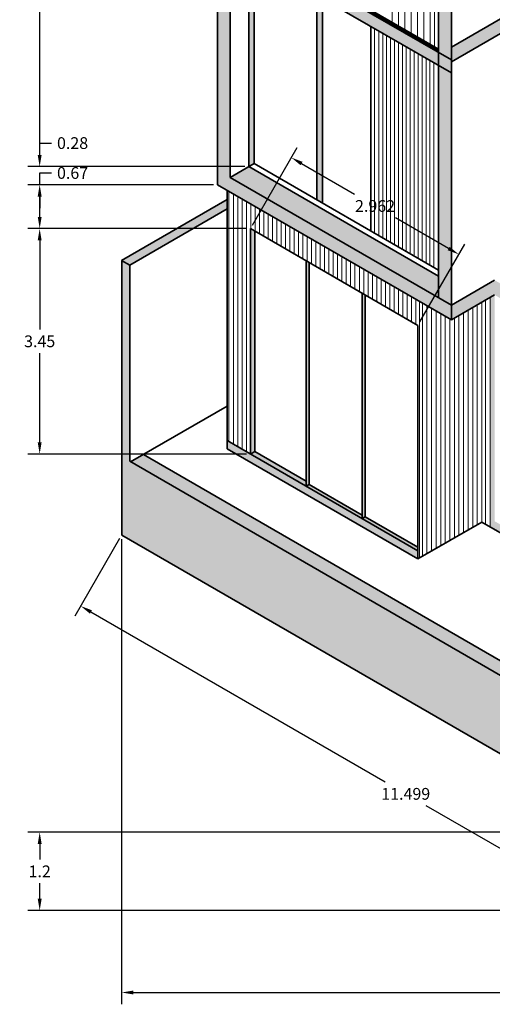
# Model space of a CAD drawing. Units: metres. Extents: x 26125 to 52281, y 14233 to 28508.
# Tile 1 of 4: x 26125.05 to 26132.29, y 14233.46 to 14248.53. Entities that reach past the tile are written whole.
import ezdxf

# ---------------------------------------------------------------- set-up
doc = ezdxf.new("R2010")
doc.units = ezdxf.units.M
for name, color, linetype, lineweight in [('A-ANNO-DIMS', 2, 'Continuous', 18), ('A-ELEV', 7, 'Continuous', 18), ('A-ELEV-CLAD', 30, 'Continuous', 13), ('A-ELEV-PATT', 32, 'Continuous', 13), ('A-WALL', 7, 'Continuous', 35), ('A-WALL-PATT', 9, 'Continuous', 13)]:
    doc.layers.add(name, color=color, linetype=linetype, lineweight=lineweight)
doc.styles.get("Standard").update_dxf_attribs({"font": 'arial.ttf'})
doc.dimstyles.get("Standard").update_dxf_attribs({"dimtxt": 0.18, "dimasz": 0.18, "dimexe": 0.18, "dimexo": 0.0625, "dimgap": 0.09, "dimtad": 0, "dimtih": 1, "dimtoh": 1, "dimdec": 4, "dimzin": 0, "dimdsep": 46, "dimtxsty": 'Standard', "dimcen": 0.09, "dimadec": 0, "dimazin": 0, "dimtfac": 1, "dimtdec": 4, "dimtofl": 0, "dimtmove": 0, "dimatfit": 3, "dimfxl": 1, "dimtolj": 1, "dimtzin": 0, "dimarcsym": 0})

# ---------------------------------------------------------------- blocks, each defined once
blk = doc.blocks.new('*D10')
at = {"layer": 'A-ANNO-DIMS', "color": 0, "lineweight": -2, "transparency": 16777216}
for p, q in [((26148.791, 14241.887), (26148.791, 14233.458)), ((26126.609, 14240.579), (26126.609, 14233.458)), ((26126.789, 14233.638), (26137.305, 14233.638)), ((26148.611, 14233.638), (26138.096, 14233.638))]:
    blk.add_line(p, q, dxfattribs=at)
at = {"layer": 'A-ANNO-DIMS', "color": 0, "transparency": 16777216}
for points in [[(26126.789, 14233.668), (26126.789, 14233.608), (26126.609, 14233.638)], [(26148.611, 14233.668), (26148.611, 14233.608), (26148.791, 14233.638)]]:
    blk.add_solid(points, dxfattribs=at)
at = {"layer": 'Defpoints', "color": 0, "transparency": 16777216}
for p in [(26148.791, 14241.95), (26126.609, 14240.642), (26148.791, 14233.638)]:
    blk.add_point(p, dxfattribs=at)
at = {"layer": 'A-ANNO-DIMS', "color": 0, "transparency": 16777216, "insert": (26137.7, 14233.638), "char_height": 0.18, "attachment_point": 5}
blk.add_mtext('\\A1;22.18', dxfattribs=at)
blk = doc.blocks.new('*D12')
at = {"layer": 'A-ANNO-DIMS', "color": 0, "lineweight": -2, "transparency": 16777216}
for p, q in [((26126.578, 14240.588), (26125.892, 14239.399)), ((26126.138, 14239.465), (26130.646, 14236.862)), ((26135.784, 14233.896), (26131.276, 14236.498)), ((26136.536, 14234.838), (26135.85, 14233.65))]:
    blk.add_line(p, q, dxfattribs=at)
at = {"layer": 'A-ANNO-DIMS', "color": 0, "transparency": 16777216}
for points in [[(26126.153, 14239.491), (26126.123, 14239.439), (26125.982, 14239.555)], [(26135.799, 14233.922), (26135.769, 14233.87), (26135.94, 14233.806)]]:
    blk.add_solid(points, dxfattribs=at)
at = {"layer": 'Defpoints', "color": 0, "transparency": 16777216}
for p in [(26126.609, 14240.642), (26125.982, 14239.555), (26136.568, 14234.893)]:
    blk.add_point(p, dxfattribs=at)
at = {"layer": 'A-ANNO-DIMS', "color": 0, "transparency": 16777216, "insert": (26130.961, 14236.68), "char_height": 0.18, "attachment_point": 5}
blk.add_mtext('\\A1;11.499', dxfattribs=at)
blk = doc.blocks.new('*D14')
at = {"layer": 'A-ANNO-DIMS', "color": 0, "lineweight": -2, "transparency": 16777216}
for p, q in [((26136.505, 14236.093), (26125.173, 14236.093)), ((26125.353, 14235.913), (26125.353, 14235.673)), ((26125.353, 14235.073), (26125.353, 14235.312)), ((26136.505, 14234.893), (26125.173, 14234.893))]:
    blk.add_line(p, q, dxfattribs=at)
at = {"layer": 'A-ANNO-DIMS', "color": 0, "transparency": 16777216}
for points in [[(26125.323, 14235.913), (26125.383, 14235.913), (26125.353, 14236.093)], [(26125.323, 14235.073), (26125.383, 14235.073), (26125.353, 14234.893)]]:
    blk.add_solid(points, dxfattribs=at)
at = {"layer": 'Defpoints', "color": 0, "transparency": 16777216}
for p in [(26125.353, 14236.093), (26136.568, 14236.093), (26136.568, 14234.893)]:
    blk.add_point(p, dxfattribs=at)
at = {"layer": 'A-ANNO-DIMS', "color": 0, "transparency": 16777216, "insert": (26125.353, 14235.493), "char_height": 0.18, "attachment_point": 5}
blk.add_mtext('\\A1;1.2', dxfattribs=at)
blk = doc.blocks.new('*D23')
at = {"layer": 'A-ANNO-DIMS', "color": 0, "lineweight": -2, "transparency": 16777216}
for p, q in [((26128.519, 14245.334), (26125.173, 14245.334)), ((26125.353, 14245.154), (26125.353, 14243.791)), ((26125.353, 14242.063), (26125.353, 14243.427)), ((26128.519, 14241.883), (26125.173, 14241.883))]:
    blk.add_line(p, q, dxfattribs=at)
at = {"layer": 'A-ANNO-DIMS', "color": 0, "transparency": 16777216}
for points in [[(26125.323, 14245.154), (26125.383, 14245.154), (26125.353, 14245.334)], [(26125.323, 14242.063), (26125.383, 14242.063), (26125.353, 14241.883)]]:
    blk.add_solid(points, dxfattribs=at)
at = {"layer": 'Defpoints', "color": 0, "transparency": 16777216}
for p in [(26125.353, 14245.334), (26128.581, 14245.334), (26128.581, 14241.883)]:
    blk.add_point(p, dxfattribs=at)
at = {"layer": 'A-ANNO-DIMS', "color": 0, "transparency": 16777216, "insert": (26125.353, 14243.609), "char_height": 0.18, "attachment_point": 5}
blk.add_mtext('\\A1;3.45', dxfattribs=at)
blk = doc.blocks.new('*D24')
at = {"layer": 'A-ANNO-DIMS', "color": 0, "lineweight": -2, "transparency": 16777216}
for p, q in [((26125.35337, 14246.006223), (26125.35337, 14246.186223)), ((26125.35337, 14246.186223), (26125.53337, 14246.186223)), ((26128.013551, 14246.006223), (26125.17337, 14246.006223)), ((26125.35337, 14245.514375), (26125.35337, 14245.826223)), ((26128.518849, 14245.334375), (26125.17337, 14245.334375))]:
    blk.add_line(p, q, dxfattribs=at)
at = {"layer": 'A-ANNO-DIMS', "color": 0, "transparency": 16777216}
for points in [[(26125.32337, 14245.826223), (26125.38337, 14245.826223), (26125.35337, 14246.006223)], [(26125.32337, 14245.514375), (26125.38337, 14245.514375), (26125.35337, 14245.334375)]]:
    blk.add_solid(points, dxfattribs=at)
at = {"layer": 'Defpoints', "color": 0, "transparency": 16777216}
for p in [(26125.35337, 14246.006223), (26128.076051, 14246.006223), (26128.581349, 14245.334375)]:
    blk.add_point(p, dxfattribs=at)
at = {"layer": 'A-ANNO-DIMS', "color": 0, "transparency": 16777216, "insert": (26125.857149, 14246.186223), "char_height": 0.18, "attachment_point": 5}
blk.add_mtext('\\A1;0.67', dxfattribs=at)
blk = doc.blocks.new('*D25')
at = {"layer": 'A-ANNO-DIMS', "color": 0, "lineweight": -2, "transparency": 16777216}
for p, q in [((26125.353, 14246.464), (26125.353, 14246.644)), ((26125.353, 14246.644), (26125.533, 14246.644)), ((26128.496, 14246.284), (26125.173, 14246.284)), ((26128.014, 14246.006), (26125.173, 14246.006)), ((26125.353, 14245.826), (26125.353, 14245.646))]:
    blk.add_line(p, q, dxfattribs=at)
at = {"layer": 'A-ANNO-DIMS', "color": 0, "transparency": 16777216}
for points in [[(26125.323, 14246.464), (26125.383, 14246.464), (26125.353, 14246.284)], [(26125.323, 14245.826), (26125.383, 14245.826), (26125.353, 14246.006)]]:
    blk.add_solid(points, dxfattribs=at)
at = {"layer": 'Defpoints', "color": 0, "transparency": 16777216}
for p in [(26125.353, 14246.284), (26128.558, 14246.284), (26128.076, 14246.006)]:
    blk.add_point(p, dxfattribs=at)
at = {"layer": 'A-ANNO-DIMS', "color": 0, "transparency": 16777216, "insert": (26125.857, 14246.644), "char_height": 0.18, "attachment_point": 5}
blk.add_mtext('\\A1;0.28', dxfattribs=at)
blk = doc.blocks.new('*D26')
at = {"layer": 'A-ANNO-DIMS', "color": 0, "lineweight": -2, "transparency": 16777216}
for p, q in [((26128.496, 14252.42), (26125.173, 14252.42)), ((26125.353, 14252.24), (26125.353, 14249.534)), ((26125.353, 14246.464), (26125.353, 14249.17)), ((26128.496, 14246.284), (26125.173, 14246.284))]:
    blk.add_line(p, q, dxfattribs=at)
at = {"layer": 'A-ANNO-DIMS', "color": 0, "transparency": 16777216}
for points in [[(26125.323, 14252.24), (26125.383, 14252.24), (26125.353, 14252.42)], [(26125.323, 14246.464), (26125.383, 14246.464), (26125.353, 14246.284)]]:
    blk.add_solid(points, dxfattribs=at)
at = {"layer": 'Defpoints', "color": 0, "transparency": 16777216}
for p in [(26125.353, 14252.42), (26128.558, 14252.42), (26128.558, 14246.284)]:
    blk.add_point(p, dxfattribs=at)
at = {"layer": 'A-ANNO-DIMS', "color": 0, "transparency": 16777216, "insert": (26125.353, 14249.352), "char_height": 0.18, "attachment_point": 5}
blk.add_mtext('\\A1;6.136', dxfattribs=at)
blk = doc.blocks.new('*D28')
at = {"layer": 'A-ANNO-DIMS', "color": 0, "lineweight": -2, "transparency": 16777216}
for p, q in [((26128.613, 14245.389), (26129.299, 14246.577)), ((26129.365, 14246.331), (26130.176, 14245.863)), ((26131.618, 14245.03), (26130.806, 14245.499)), ((26131.178, 14243.908), (26131.864, 14245.096))]:
    blk.add_line(p, q, dxfattribs=at)
at = {"layer": 'A-ANNO-DIMS', "color": 0, "transparency": 16777216}
for points in [[(26129.38, 14246.357), (26129.35, 14246.305), (26129.209, 14246.421)], [(26131.633, 14245.056), (26131.603, 14245.004), (26131.774, 14244.94)]]:
    blk.add_solid(points, dxfattribs=at)
at = {"layer": 'Defpoints', "color": 0, "transparency": 16777216}
for p in [(26128.581, 14245.334), (26131.774, 14244.94), (26131.146, 14243.853)]:
    blk.add_point(p, dxfattribs=at)
at = {"layer": 'A-ANNO-DIMS', "color": 0, "transparency": 16777216, "insert": (26130.491, 14245.681), "char_height": 0.18, "attachment_point": 5}
blk.add_mtext('\\A1;2.962', dxfattribs=at)

msp = doc.modelspace()

# ---------------------------------------------------------------- hatches: boundary and pattern name
at = {"layer": 'A-ELEV-PATT'}
h = msp.add_hatch(color=256, dxfattribs=at)
h.dxf.hatch_style = 1
h.paths.add_polyline_path([(26128.6368, 14249.6632), (26128.6368, 14249.4632), (26131.4647, 14247.8305), (26131.4647, 14248.0305)])
h.paths.add_polyline_path([(26129.6878, 14248.8564), (26129.5992, 14248.9076), (26129.5992, 14245.7744), (26129.6878, 14245.7232)])
h.paths.add_polyline_path([(26128.6368, 14249.4632), (26128.558, 14249.5087), (26128.558, 14246.2845), (26128.6368, 14246.33)])
h.paths.add_polyline_path([(26128.6368, 14249.6632), (26128.558, 14249.7087), (26128.558, 14249.5087), (26128.6368, 14249.4632)])
h.paths.add_polyline_path([(26128.6368, 14252.3748), (26128.558, 14252.4203), (26128.558, 14249.7087), (26128.6368, 14249.6632)])
h.paths.add_polyline_path([(26128.651, 14245.2941), (26128.5813, 14245.3344), (26128.5813, 14241.8829), (26128.651, 14241.9232)])
h.paths.add_polyline_path([(26128.651, 14241.9232), (26128.5813, 14241.8829), (26129.4364, 14241.3893), (26129.4364, 14241.4697)])
h.paths.add_polyline_path([(26129.4797, 14241.4143), (26129.4364, 14241.3893), (26130.2914, 14240.8956), (26130.2914, 14240.9456)])
h.paths.add_polyline_path([(26130.3373, 14240.9221), (26130.2914, 14240.8956), (26131.1464, 14240.402), (26131.1464, 14240.455)])
h.paths.add_polyline_path([(26130.3373, 14244.3206), (26130.2914, 14244.3471), (26130.2914, 14240.8956), (26130.3373, 14240.9221)])
h.paths.add_polyline_path([(26129.4797, 14244.8157), (26129.4364, 14244.8407), (26129.4364, 14241.3893), (26129.4797, 14241.4143)])
h.paths.add_polyline_path([(26135.2508, 14242.6282), (26135.1411, 14242.6915), (26135.1411, 14239.2275), (26135.2508, 14239.2908)])
h.paths.add_polyline_path([(26133.8091, 14243.4606), (26133.706, 14243.5201), (26133.706, 14240.056), (26133.8091, 14240.1155)])
h.paths.add_polyline_path([(26132.3223, 14244.3189), (26132.2523, 14244.2785), (26132.2523, 14240.7692), (26132.3223, 14240.7288)])
at = {"layer": 'A-WALL-PATT'}
h = msp.add_hatch(color=256, dxfattribs=at)
h.dxf.hatch_style = 1
h.paths.add_polyline_path([(26132.7127, 14248.4963), (26132.7127, 14248.7223), (26131.6604, 14248.1148), (26131.6604, 14247.8888)])
h.paths.add_polyline_path([(26132.7127, 14248.7223), (26132.7127, 14248.4963), (26136.7743, 14246.1513), (26136.7743, 14246.3773)])
h.paths.add_polyline_path([(26145.7774, 14251.3492), (26145.7774, 14250.8522), (26145.9732, 14250.9652), (26145.9732, 14251.6882), (26145.9732, 14252.3156), (26145.7774, 14252.4288), (26145.7774, 14251.5752), (26136.7743, 14246.3773), (26136.7743, 14246.1513), (26136.97, 14246.2643), (26136.97, 14246.1509), (26137.1658, 14246.2639), (26137.1658, 14246.3773)])
h.paths.add_polyline_path([(26135.3545, 14249.1132), (26135.1588, 14249.0002), (26138.2381, 14247.2224), (26138.4338, 14247.3354)])
h.paths.add_polyline_path([(26135.3545, 14252.0261), (26135.1588, 14252.1391), (26135.1588, 14249.0002), (26135.3545, 14249.1132)])
h.paths.add_polyline_path([(26137.9254, 14251.8375), (26137.7296, 14251.7245), (26137.7296, 14250.6548), (26137.9254, 14250.7678)], flags=17)
h.paths.add_polyline_path([(26144.9726, 14252.8939), (26144.9726, 14254.6106), (26144.7764, 14254.4973), (26144.7764, 14252.7806), (26145.7774, 14252.2026), (26145.7774, 14252.4288)])
h.paths.add_polyline_path([(26147.5095, 14248.6232), (26147.5095, 14242.6232), (26147.7052, 14242.7362), (26147.7052, 14248.9622), (26136.1883, 14242.3129), (26136.1883, 14242.0869), (26136.97, 14242.5383), (26136.97, 14242.3123), (26137.1658, 14242.4253), (26137.1658, 14242.6513)])
h.paths.add_polyline_path([(26145.9732, 14249.2872), (26145.7774, 14249.1742), (26145.7774, 14247.8492), (26145.9732, 14247.9622)], flags=17)
h.paths.add_polyline_path([(26145.5817, 14254.9622), (26145.5817, 14254.7362), (26145.7774, 14254.8492), (26145.7774, 14255.5272), (26145.5817, 14255.4142), (26145.5817, 14255.1882), (26141.4857, 14252.8234), (26141.4857, 14252.5974)])
h.paths.add_polyline_path([(26140.5667, 14258.3096), (26140.5667, 14258.0836), (26145.5817, 14255.1882), (26145.5817, 14255.4142)])
h.paths.add_polyline_path([(26140.7524, 14259.0772), (26140.7524, 14259.3025), (26137.3207, 14257.3212), (26137.5157, 14257.2086)])
h.paths.add_polyline_path([(26138.0751, 14255.9856), (26138.3349, 14256.1356), (26138.5947, 14255.9856), (26138.5947, 14256.5856), (26138.0751, 14256.2856), (26134.148, 14254.0183), (26134.4078, 14253.8683)])
h.paths.add_polyline_path([(26140.5667, 14258.0836), (26140.5667, 14258.3096), (26140.7524, 14258.4285), (26140.7524, 14259.0772), (26137.5157, 14257.2086), (26138.2834, 14256.7653)])
h.paths.add_polyline_path([(26145.1083, 14255.9136), (26145.0216, 14255.8636), (26144.9721, 14255.8922), (26144.9721, 14255.9922), (26144.9373, 14256.0123), (26144.8507, 14255.9623), (26144.8012, 14255.9909), (26144.8012, 14256.0909), (26144.7664, 14256.1109), (26144.6798, 14256.0609), (26144.6303, 14256.0896), (26144.6303, 14256.1896), (26144.5955, 14256.2096), (26144.5089, 14256.1596), (26144.4594, 14256.1882), (26144.4594, 14256.2882), (26144.4246, 14256.3083), (26144.338, 14256.2583), (26144.2885, 14256.2869), (26144.2885, 14256.3869), (26144.2537, 14256.407), (26144.1671, 14256.357), (26144.1176, 14256.3856), (26144.1176, 14256.4856), (26144.0828, 14256.5056), (26143.9962, 14256.4556), (26143.9466, 14256.4842), (26143.9466, 14256.5842), (26143.9119, 14256.6043), (26143.8253, 14256.5543), (26143.7757, 14256.5829), (26143.7757, 14256.6829), (26143.741, 14256.703), (26143.6544, 14256.653), (26143.6048, 14256.6816), (26143.6048, 14256.7816), (26143.5701, 14256.8017), (26143.4835, 14256.7517), (26143.4339, 14256.7803), (26143.4339, 14256.8803), (26143.3992, 14256.9003), (26143.3126, 14256.8503), (26143.263, 14256.8789), (26143.263, 14256.9789), (26143.2283, 14256.999), (26143.1417, 14256.949), (26143.0921, 14256.9776), (26143.0921, 14257.0776), (26143.0573, 14257.0977), (26142.9707, 14257.0477), (26142.9212, 14257.0763), (26142.9212, 14257.1763), (26142.8864, 14257.1964), (26142.7998, 14257.1464), (26142.7503, 14257.175), (26142.7503, 14257.275), (26142.7155, 14257.295), (26142.6289, 14257.245), (26142.5794, 14257.2736), (26142.5794, 14257.3736), (26142.5446, 14257.3937), (26142.458, 14257.3437), (26142.4085, 14257.3723), (26142.4085, 14257.4723), (26142.3737, 14257.4924), (26142.2871, 14257.4424), (26142.2376, 14257.471), (26142.2376, 14257.571), (26142.2322, 14257.5741), (26142.1456, 14257.5241), (26142.0961, 14257.5527), (26142.0961, 14257.6527), (26142.0613, 14257.6727), (26141.9747, 14257.6227), (26141.9252, 14257.6514), (26141.9252, 14257.7514), (26141.8904, 14257.7714), (26141.8038, 14257.7214), (26141.7542, 14257.75), (26141.7542, 14257.85), (26141.7195, 14257.8701), (26141.6329, 14257.8201), (26141.5833, 14257.8487), (26141.5833, 14257.9487), (26141.5486, 14257.9688), (26141.462, 14257.9188), (26141.4124, 14257.9474), (26141.4124, 14258.0474), (26141.3777, 14258.0674), (26141.2911, 14258.0174), (26141.2415, 14258.0461), (26141.2415, 14258.1461), (26141.2068, 14258.1661), (26141.1202, 14258.1161), (26141.0706, 14258.1447), (26141.0706, 14258.2447), (26141.0359, 14258.2648), (26140.9493, 14258.2148), (26140.8997, 14258.2434), (26140.8997, 14258.3434), (26140.8885, 14258.3499), (26140.8019, 14258.2999), (26140.7524, 14258.3285), (26140.7524, 14258.4285), (26140.5667, 14258.3096), (26145.5817, 14255.4142), (26145.7774, 14255.5272)])
h.paths.add_polyline_path([(26141.4857, 14254.3165), (26141.3093, 14254.2146), (26141.3093, 14252.4955), (26141.4857, 14252.5974)])
h.paths.add_polyline_path([(26140.2525, 14255.0285), (26140.0568, 14254.9155), (26141.29, 14254.2035), (26141.4857, 14254.3165)])
h = msp.add_hatch(color=256, dxfattribs=at)
h.dxf.hatch_style = 1
h.paths.add_polyline_path([(26131.6604, 14251.2489), (26128.0761, 14253.3183), (26128.0761, 14246.0062), (26131.6604, 14243.9368), (26131.6604, 14244.1628), (26128.2718, 14246.1192), (26128.2718, 14252.9793), (26131.4647, 14251.1359), (26131.4647, 14248.0305), (26131.6604, 14247.9175)])
h.paths.add_polyline_path([(26131.6604, 14245.2298), (26131.6604, 14247.7175), (26131.4647, 14247.8305), (26131.4647, 14244.2758), (26131.6604, 14244.1628)], flags=17)
h = msp.add_hatch(color=256, dxfattribs=at)
h.dxf.hatch_style = 1
h.paths.add_polyline_path([(26131.6604, 14247.9175), (26131.4647, 14248.0305), (26131.4647, 14247.8305), (26131.6604, 14247.7175)])
h = msp.add_hatch(color=256, dxfattribs=at)
h.dxf.hatch_style = 1
h.paths.add_polyline_path([(26126.9422, 14241.8758), (26126.7465, 14241.7628), (26136.5676, 14236.0925), (26136.7633, 14236.2055)])
h.paths.add_polyline_path([(26126.7465, 14241.7628), (26126.7318, 14241.7712), (26126.7318, 14244.7755), (26126.6095, 14244.8461), (26126.6095, 14240.6418), (26136.5676, 14234.8925), (26136.5676, 14236.0925)])
h.paths.add_polyline_path([(26138.4953, 14236.3449), (26138.4953, 14237.2055), (26136.7633, 14236.2055), (26136.7633, 14235.0055), (26138.2239, 14235.8488), (26138.1257, 14235.9055), (26138.1257, 14236.1315)])
h.paths.add_polyline_path([(26140.7034, 14237.2803), (26147.9009, 14241.4358), (26147.9009, 14241.6618), (26147.7052, 14241.5488), (26140.6052, 14237.4496), (26138.2239, 14236.0748), (26138.2239, 14235.8488)])
h.paths.add_polyline_path([(26140.6052, 14237.4496), (26142.2637, 14238.4072), (26142.2637, 14238.5206), (26138.6911, 14236.4579), (26138.6911, 14236.3445)], flags=17)
h.paths.add_polyline_path([(26138.4953, 14236.2315), (26138.4953, 14236.3449), (26138.1257, 14236.1315), (26138.2239, 14236.0748)], flags=17)
h.paths.add_polyline_path([(26138.2239, 14236.0748), (26138.1257, 14236.1315), (26138.1257, 14235.9055), (26138.2239, 14235.8488)], flags=17)
h.paths.add_polyline_path([(26136.7633, 14236.2055), (26136.5676, 14236.0925), (26136.5676, 14234.8925), (26136.7633, 14235.0055)])
h.paths.add_polyline_path([(26138.4953, 14237.2055), (26138.2996, 14237.3185), (26136.5676, 14236.3185), (26136.7633, 14236.2055)])
h.paths.add_polyline_path([(26128.558, 14246.2845), (26128.2718, 14246.1192), (26131.4647, 14244.2758), (26131.4647, 14244.6063)])
h.paths.add_polyline_path([(26128.2234, 14245.6367), (26128.2234, 14245.7792), (26126.6095, 14244.8474), (26126.6095, 14244.8461), (26126.7318, 14244.7755)])
h = msp.add_hatch(color=256, dxfattribs=at)
h.dxf.hatch_style = 1
h.paths.add_polyline_path([(26132.3223, 14244.3189), (26132.3223, 14244.5449), (26131.6604, 14244.1628), (26131.6604, 14243.9368)])
h.paths.add_polyline_path([(26132.3223, 14244.5449), (26132.3223, 14244.3189), (26136.1883, 14242.0869), (26136.1883, 14242.3129)])
h.paths.add_polyline_path([(26132.3223, 14240.8549), (26132.3223, 14240.7288), (26136.97, 14238.0454), (26136.97, 14238.1715)])
h.paths.add_polyline_path([(26128.2234, 14242.0896), (26128.2234, 14241.9635), (26131.1464, 14240.2759), (26131.1464, 14240.402)])

# ---------------------------------------------------------------- linework, layer by layer
at = {"layer": 'A-ELEV'}
for p in [(26129.2226, 14245.3443), (26129.4364, 14244.8407), (26130.2914, 14244.3471)]:
    msp.add_point(p, dxfattribs=at)
at = {"layer": 'A-ELEV-CLAD'}
for p, q in [((26130.7506, 14248.4938), (26130.7506, 14251.1544)), ((26130.8482, 14248.4374), (26130.8482, 14251.098)), ((26130.9459, 14248.381), (26130.9459, 14251.0416)), ((26131.0436, 14248.3246), (26131.0436, 14250.9853)), ((26131.1412, 14248.2682), (26131.1412, 14250.9289)), ((26131.2389, 14248.2118), (26131.2389, 14250.8725)), ((26131.3366, 14248.1554), (26131.3366, 14250.8161)), ((26131.3997, 14248.119), (26131.3997, 14250.7796)), ((26130.4806, 14245.2654), (26130.4806, 14248.3986)), ((26130.5477, 14245.2267), (26130.5477, 14248.3599)), ((26130.608, 14245.1919), (26130.608, 14248.3251)), ((26130.6684, 14245.1571), (26130.6684, 14248.2903)), ((26130.7287, 14245.1222), (26130.7287, 14248.2554)), ((26130.789, 14245.0874), (26130.789, 14248.2206)), ((26130.8493, 14245.0526), (26130.8493, 14248.1858)), ((26130.9097, 14245.0177), (26130.9097, 14248.1509)), ((26130.97, 14244.9829), (26130.97, 14248.1161)), ((26131.0303, 14244.9481), (26131.0303, 14248.0813)), ((26131.0906, 14244.9133), (26131.0906, 14248.0465)), ((26131.151, 14244.8784), (26131.151, 14248.0116)), ((26131.2113, 14244.8436), (26131.2113, 14247.9768)), ((26131.2716, 14244.8088), (26131.2716, 14247.942)), ((26131.3319, 14244.7739), (26131.3319, 14247.9072)), ((26131.3923, 14244.7391), (26131.3923, 14247.8723)), ((26128.2496, 14242.0745), (26128.2496, 14245.906)), ((26128.3214, 14242.033), (26128.3214, 14245.8645)), ((26128.3879, 14241.9946), (26128.3879, 14245.8262)), ((26128.4544, 14241.9562), (26128.4544, 14245.7878)), ((26128.5208, 14241.9179), (26128.5208, 14245.7494)), ((26128.5873, 14245.3309), (26128.5873, 14245.7111)), ((26128.6538, 14245.2926), (26128.6538, 14245.6727)), ((26128.7202, 14245.2542), (26128.7202, 14245.6343)), ((26128.7867, 14245.2158), (26128.7867, 14245.5959)), ((26128.8531, 14245.1775), (26128.8531, 14245.5576)), ((26128.9196, 14245.1391), (26128.9196, 14245.5192)), ((26128.9861, 14245.1007), (26128.9861, 14245.4808)), ((26129.0525, 14245.0623), (26129.0525, 14245.4425)), ((26129.119, 14245.024), (26129.119, 14245.4041)), ((26129.1855, 14244.9856), (26129.1855, 14245.3657)), ((26129.2519, 14244.9472), (26129.2519, 14245.3273)), ((26129.2519, 14244.9472), (26129.2519, 14245.3273)), ((26129.3184, 14244.9088), (26129.3184, 14245.289)), ((26129.3848, 14244.8705), (26129.3848, 14245.2506)), ((26129.4513, 14244.8321), (26129.4513, 14245.2122)), ((26129.5178, 14244.7937), (26129.5178, 14245.1738)), ((26129.5842, 14244.7554), (26129.5842, 14245.1355)), ((26129.6507, 14244.717), (26129.6507, 14245.0971)), ((26129.7172, 14244.6786), (26129.7172, 14245.0587)), ((26129.7836, 14244.6402), (26129.7836, 14245.0204)), ((26129.8501, 14244.6019), (26129.8501, 14244.982)), ((26129.9165, 14244.5635), (26129.9165, 14244.9436)), ((26129.983, 14244.5251), (26129.983, 14244.9052)), ((26130.0495, 14244.4868), (26130.0495, 14244.8669)), ((26130.1159, 14244.4484), (26130.1159, 14244.8285)), ((26130.1824, 14244.41), (26130.1824, 14244.7901)), ((26130.1836, 14244.4093), (26130.1836, 14244.7894)), ((26130.2501, 14244.3709), (26130.2501, 14244.751)), ((26130.3165, 14244.3326), (26130.3165, 14244.7127)), ((26130.383, 14244.2942), (26130.383, 14244.6743)), ((26130.4495, 14244.2558), (26130.4495, 14244.6359)), ((26130.5159, 14244.2174), (26130.5159, 14244.5976)), ((26130.5824, 14244.1791), (26130.5824, 14244.5592)), ((26130.6489, 14244.1407), (26130.6489, 14244.5208)), ((26130.7153, 14244.1023), (26130.7153, 14244.4824)), ((26130.7818, 14244.064), (26130.7818, 14244.4441)), ((26130.8482, 14244.0256), (26130.8482, 14244.4057)), ((26130.9147, 14243.9872), (26130.9147, 14244.3673)), ((26130.9812, 14243.9488), (26130.9812, 14244.329)), ((26131.0476, 14243.9105), (26131.0476, 14244.2906)), ((26131.1141, 14243.8721), (26131.1141, 14244.2522)), ((26131.1704, 14240.2897), (26131.1704, 14244.2197)), ((26132.1266, 14244.2059), (26132.1266, 14240.8418)), ((26132.1823, 14244.2381), (26132.1823, 14240.8096)), ((26132.2523, 14244.2785), (26132.2523, 14240.7692)), ((26131.2164, 14244.1931), (26131.2164, 14240.3163)), ((26131.2865, 14244.1527), (26131.2865, 14240.3567)), ((26131.3565, 14244.1123), (26131.3565, 14240.3971)), ((26131.4265, 14244.0719), (26131.4265, 14240.4376)), ((26131.9166, 14244.0847), (26131.9166, 14240.7205)), ((26131.9866, 14244.1251), (26131.9866, 14240.7609)), ((26132.0566, 14244.1655), (26132.0566, 14240.8014)), ((26131.4965, 14244.0314), (26131.4965, 14240.478)), ((26131.5665, 14243.991), (26131.5665, 14240.5184)), ((26131.6365, 14243.9506), (26131.6365, 14240.5588)), ((26131.7065, 14243.9634), (26131.7065, 14240.5992)), ((26131.7765, 14244.0038), (26131.7765, 14240.6397)), ((26131.8466, 14244.0443), (26131.8466, 14240.6801))]:
    msp.add_line(p, q, dxfattribs=at)
at = {"layer": 'A-WALL'}
for p, q in [((26128.0761, 14253.3183), (26128.0761, 14246.0062)), ((26128.2718, 14252.9793), (26128.2718, 14246.1192)), ((26128.558, 14252.4203), (26128.558, 14246.2845)), ((26128.6368, 14252.3748), (26128.6368, 14246.33)), ((26131.4647, 14251.1359), (26131.4647, 14244.2758)), ((26131.6604, 14251.2489), (26131.6604, 14244.1628)), ((26128.558, 14249.7087), (26131.6604, 14247.9175)), ((26128.6598, 14249.6765), (26131.4647, 14248.0571)), ((26128.681, 14249.6887), (26131.4647, 14248.0815)), ((26128.558, 14249.5087), (26131.6604, 14247.7175)), ((26129.5992, 14248.9076), (26129.5992, 14245.7744)), ((26129.6878, 14248.8564), (26129.6878, 14245.7232)), ((26132.7127, 14248.7223), (26131.6604, 14248.1148)), ((26130.4287, 14245.4352), (26130.4287, 14248.4286)), ((26130.4287, 14245.2954), (26130.4287, 14248.4286)), ((26132.7127, 14248.4963), (26131.6604, 14247.8888)), ((26128.2718, 14246.1192), (26128.6368, 14246.33)), ((26128.6368, 14246.33), (26131.4647, 14244.6973)), ((26128.558, 14246.2845), (26131.4647, 14244.6063)), ((26131.6604, 14244.1628), (26128.2718, 14246.1192)), ((26131.6604, 14243.9368), (26128.0761, 14246.0062)), ((26128.2234, 14245.9212), (26128.2234, 14241.9635)), ((26128.2234, 14245.7792), (26126.6084, 14244.8467)), ((26128.2234, 14245.6367), (26126.7318, 14244.7755)), ((26128.5813, 14245.3344), (26128.5813, 14241.8829)), ((26131.1464, 14243.8534), (26128.5813, 14245.3344)), ((26128.651, 14245.2941), (26128.651, 14241.9232)), ((26131.6604, 14243.9368), (26131.6604, 14245.2298)), ((26126.7318, 14244.7755), (26126.6084, 14244.8467)), ((26126.6095, 14240.6418), (26126.6095, 14244.8461)), ((26129.4364, 14244.8407), (26129.4364, 14241.3893)), ((26129.4797, 14244.8157), (26129.4797, 14241.4143)), ((26126.7318, 14241.7712), (26126.7318, 14244.7755)), ((26132.3223, 14244.5449), (26131.6604, 14244.1628)), ((26130.2914, 14244.3471), (26130.2914, 14240.8956)), ((26130.3373, 14244.3206), (26130.3373, 14240.9221)), ((26132.3223, 14244.3189), (26131.6604, 14243.9368)), ((26131.1464, 14243.8534), (26131.1464, 14240.2759)), ((26126.7465, 14241.7628), (26128.2234, 14242.6155)), ((26131.1464, 14240.402), (26128.2234, 14242.0896)), ((26131.1464, 14240.2759), (26128.2234, 14241.9635)), ((26136.7633, 14236.2055), (26126.9422, 14241.8758)), ((26128.5813, 14241.8829), (26128.651, 14241.9232)), ((26128.651, 14241.9232), (26129.4364, 14241.4697)), ((26136.5676, 14236.0925), (26126.7318, 14241.7712)), ((26129.4364, 14241.3893), (26129.4797, 14241.4143)), ((26129.4797, 14241.4143), (26130.2914, 14240.9456)), ((26130.2914, 14240.8956), (26130.3373, 14240.9221)), ((26130.3373, 14240.9221), (26131.1464, 14240.455)), ((26131.1464, 14240.2759), (26132.1266, 14240.8418)), ((26132.1266, 14240.8418), (26138.2643, 14237.2982)), ((26136.5676, 14234.8925), (26126.6095, 14240.6418))]:
    msp.add_line(p, q, dxfattribs=at)

# ---------------------------------------------------------------- dimensions: what is measured, and where the dimension line sits
at = {"layer": 'A-ANNO-DIMS'}
for base, p1, p2, angle, override, picture, middle in [((26125.3534, 14252.4203), (26128.558, 14246.2845), (26128.558, 14252.4203), 90, {"dimdec": 3, "dimlfac": 1, "dimrnd": 0, "dimzin": 0, "dimdsep": 46, "dimlunit": 2}, '*D26', (26125.3534, 14249.3524)), ((26125.3534, 14246.2845), (26128.0761, 14246.0062), (26128.558, 14246.2845), 90, {"dimdec": 2, "dimlfac": 1, "dimrnd": 0, "dimzin": 0, "dimdsep": 46, "dimlunit": 2}, '*D25', (26125.8573, 14246.6445)), ((26131.7739, 14244.9403), (26128.5813, 14245.3344), (26131.1464, 14243.8534), 330, {"dimdec": 3, "dimlfac": 1, "dimrnd": 0, "dimzin": 0, "dimdsep": 46, "dimlunit": 2}, '*D28', (26130.4914, 14245.6808)), ((26125.3534, 14246.0062), (26128.5813, 14245.3344), (26128.0761, 14246.0062), 90, {"dimdec": 2, "dimlfac": 1, "dimrnd": 0, "dimzin": 0, "dimdsep": 46, "dimlunit": 2}, '*D24', (26125.8571, 14246.1862)), ((26125.3534, 14245.3344), (26128.5813, 14241.8829), (26128.5813, 14245.3344), 90, {"dimdec": 2, "dimlfac": 1, "dimrnd": 0, "dimzin": 0, "dimdsep": 46, "dimlunit": 2}, '*D23', (26125.3534, 14243.6087)), ((26125.982, 14239.555), (26136.5676, 14234.8925), (26126.6095, 14240.6418), 150, {"dimdec": 3, "dimlfac": 1, "dimrnd": 0, "dimzin": 0, "dimdsep": 46, "dimlunit": 2}, '*D12', (26130.961, 14236.6803)), ((26125.3534, 14236.0925), (26136.5676, 14234.8925), (26136.5676, 14236.0925), 90, {"dimdec": 1, "dimlfac": 1, "dimrnd": 0, "dimzin": 0, "dimdsep": 46, "dimlunit": 2}, '*D14', (26125.3534, 14235.4925))]:
    dim = msp.add_linear_dim(base=base, p1=p1, p2=p2, angle=angle, dimstyle='Standard', override=override, dxfattribs=at)
    dim.commit()
    dim.dimension.update_dxf_attribs({"geometry": picture, "text_midpoint": middle})
dim = msp.add_linear_dim(base=(26148.7909, 14233.6375), p1=(26126.6095, 14240.6418), p2=(26148.7909, 14241.9496), dimstyle='Standard', override={"dimdec": 2, "dimlfac": 1, "dimrnd": 0, "dimzin": 0, "dimdsep": 46, "dimlunit": 2}, dxfattribs=at)
dim.commit()
dim.dimension.update_dxf_attribs({"geometry": '*D10', "text_midpoint": (26137.7002, 14233.6375)})

doc.saveas('drawing.dxf')
